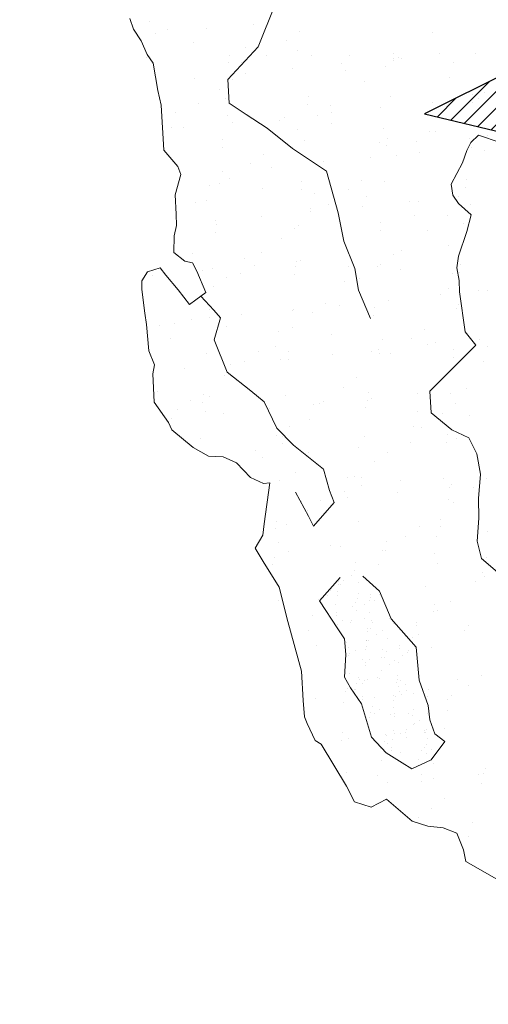
# Model space of a CAD drawing. Units: inches. Extents: x 1986 to 21484, y -1816 to 2016.
# Tile 54 of 85: x 3644.98 to 3651.09, y 1870.8 to 1883.64. Entities that reach past the tile are written whole.
import ezdxf

# ---------------------------------------------------------------- set-up
doc = ezdxf.new("R2010")
doc.units = ezdxf.units.IN
for name, color, linetype, lineweight in [('A-ANNO-DIMS', 2, 'Continuous', 18), ('L-PLNT', 84, 'Continuous', 13), ('vfolhas', 114, 'Continuous', 5)]:
    doc.layers.add(name, color=color, linetype=linetype, lineweight=lineweight)
doc.layers.add('vfolhas2', color=102, linetype='Continuous')
doc.styles.get("Standard").update_dxf_attribs({"font": 'arial.ttf'})
doc.dimstyles.new('ISO-25', dxfattribs={"dimtxt": 8, "dimasz": 2.5, "dimexe": 1.25, "dimexo": 0.625, "dimtad": 1, "dimdec": 1, "dimlunit": 3, "dimtxsty": 'Standard', "dimcen": 2.5, "dimadec": 0, "dimazin": 0, "dimtfac": 1, "dimtdec": 1, "dimtmove": 0, "dimatfit": 3, "dimfxl": 1, "dimarcsym": 0})

# ---------------------------------------------------------------- blocks, each defined once
blk = doc.blocks.new('arbusto_PB_verde_grande')
at = {"layer": 'vfolhas'}
h = blk.add_hatch(dxfattribs=at)
h.set_pattern_fill('ANSI31', color=256, scale=0.05, style=0)
h.set_pattern_definition([(45, (-2446.5133113, 50.986076), (-0.004419417382, 0.004419417382), [])])
h.paths.add_polyline_path([(-0.57219, 0.06233), (-0.7153, 0.10298), (-0.67736, 0.08107), (-0.62769, 0.01536), (-0.56347, -0.04095), (-0.26461, -0.0834), (-0.14874, -0.06595), (-0.10151, -0.05877), (-0.20418, -0.0472), (-0.40279, -0.00339)])
h.paths.add_polyline_path([(-0.56347, -0.04095), (-0.58279, -0.02401), (-0.72992, -0.09726), (-0.4334, -0.1679), (-0.41452, -0.15048), (-0.31518, -0.09101), (-0.26461, -0.0834)])
h.paths.add_polyline_path([(-0.2769, -0.47267), (-0.27429, -0.44776), (-0.16328, -0.25376), (0.02625, -0.03934), (-0.21007, -0.20995), (-0.2672, -0.24466), (-0.36485, -0.35697), (-0.42907, -0.46341), (-0.47586, -0.60425), (-0.37946, -0.57603)])
at = {"layer": 'vfolhas2'}
for p, q in [((-0.58279, -0.02401), (-0.72992, -0.09726)), ((-0.72992, -0.09726), (-0.4334, -0.1679))]:
    blk.add_line(p, q, dxfattribs=at)
blk = doc.blocks.new('PLANT-SHRUB')
for p, q in [((2184.788, 1886.333), (2184.967, 1885.753)), ((2184.967, 1885.753), (2184.886, 1885.62)), ((2184.724, 1885.539), (2184.724, 1885.539)), ((2184.886, 1885.62), (2184.799, 1885.401)), ((2184.551, 1885.444), (2184.551, 1885.444)), ((2184.799, 1885.401), (2184.88, 1885.228)), ((2184.117, 1885.152), (2184.117, 1885.152)), ((2184.88, 1885.228), (2185.013, 1885.078)), ((2183.949, 1885.045), (2183.949, 1885.045)), ((2184.011, 1885.069), (2184.011, 1885.069)), ((2184.062, 1885.039), (2184.062, 1885.039)), ((2185.013, 1885.078), (2185.117, 1884.888)), ((2184.605, 1884.968), (2184.605, 1884.968)), ((2184.813, 1884.94), (2184.813, 1884.94)), ((2185.028, 1884.913), (2185.028, 1884.913)), ((2185.117, 1884.888), (2185.163, 1884.45)), ((2184.526, 1884.674), (2184.526, 1884.674)), ((2184.387, 1884.475), (2184.095, 1884.424)), ((2184.387, 1884.475), (2184.387, 1884.475)), ((2184.654, 1884.389), (2184.387, 1884.475)), ((2184.401, 1884.538), (2184.401, 1884.538)), ((2184.607, 1884.526), (2184.607, 1884.526)), ((2184.68, 1884.594), (2184.68, 1884.594)), ((2184.095, 1884.424), (2184.121, 1884.259)), ((2184.293, 1884.388), (2184.293, 1884.388)), ((2184.377, 1884.377), (2184.377, 1884.377)), ((2184.507, 1884.36), (2184.507, 1884.36)), ((2184.691, 1884.247), (2184.654, 1884.389)), ((2185.163, 1884.45), (2185.382, 1884.392)), ((2185.163, 1884.45), (2185.163, 1884.45)), ((2185.382, 1884.392), (2185.492, 1884.19)), ((2183.986, 1884.299), (2183.986, 1884.299)), ((2184.121, 1884.259), (2184.045, 1884.082)), ((2184.235, 1884.244), (2184.235, 1884.244)), ((2184.302, 1884.287), (2184.302, 1884.287)), ((2184.338, 1884.301), (2184.338, 1884.301)), ((2184.396, 1884.3), (2184.396, 1884.3)), ((2184.755, 1884.006), (2184.691, 1884.247)), ((2185.008, 1884.304), (2185.008, 1884.304)), ((2183.16, 1884.123), (2183.16, 1884.123)), ((2183.368, 1884.095), (2183.368, 1884.095)), ((2183.795, 1884.152), (2183.795, 1884.152)), ((2184.045, 1884.082), (2183.931, 1883.93)), ((2184.17, 1884.146), (2184.17, 1884.146)), ((2184.194, 1884.14), (2184.194, 1884.14)), ((2184.199, 1884.173), (2184.199, 1884.173)), ((2184.209, 1884.162), (2184.209, 1884.162)), ((2184.612, 1884.134), (2184.612, 1884.134)), ((2185.039, 1884.149), (2185.039, 1884.149)), ((2185.492, 1884.19), (2185.428, 1883.971)), ((2183.626, 1884.044), (2183.626, 1884.044)), ((2183.693, 1884.053), (2183.693, 1884.053)), ((2183.977, 1883.99), (2183.977, 1883.99)), ((2184.011, 1884), (2184.011, 1884)), ((2184.146, 1883.993), (2184.146, 1883.993)), ((2184.229, 1883.982), (2184.229, 1883.982)), ((2184.236, 1883.981), (2184.236, 1883.981)), ((2184.359, 1883.965), (2184.359, 1883.965)), ((2184.386, 1883.992), (2184.386, 1883.992)), ((2184.416, 1884.041), (2184.416, 1884.041)), ((2184.444, 1883.954), (2184.444, 1883.954)), ((2184.651, 1884.006), (2184.651, 1884.006)), ((2184.68, 1884.033), (2184.68, 1884.033)), ((2184.755, 1884.006), (2184.755, 1884.006)), ((2184.755, 1883.727), (2184.755, 1884.006)), ((2184.871, 1884.042), (2184.871, 1884.042)), ((2185.428, 1883.971), (2185.296, 1883.345)), ((2183.421, 1883.943), (2183.421, 1883.943)), ((2183.931, 1883.93), (2183.791, 1883.613)), ((2183.861, 1883.843), (2183.861, 1883.843)), ((2184.105, 1883.844), (2184.105, 1883.844)), ((2184.173, 1883.887), (2184.173, 1883.887)), ((2184.183, 1883.832), (2184.183, 1883.832)), ((2184.491, 1883.86), (2184.491, 1883.86)), ((2184.501, 1883.904), (2184.501, 1883.904)), ((2184.576, 1883.936), (2184.576, 1883.936)), ((2184.602, 1883.826), (2184.602, 1883.826)), ((2184.603, 1883.843), (2184.603, 1883.843)), ((2184.659, 1883.926), (2184.659, 1883.926)), ((2184.671, 1883.886), (2184.671, 1883.886)), ((2184.769, 1883.911), (2184.769, 1883.911)), ((2185.312, 1883.84), (2185.312, 1883.84)), ((2183.788, 1883.776), (2183.788, 1883.776)), ((2184.323, 1883.706), (2184.323, 1883.706)), ((2184.352, 1883.733), (2184.352, 1883.733)), ((2184.552, 1883.322), (2184.755, 1883.727)), ((2183.791, 1883.613), (2183.525, 1883.271)), ((2183.967, 1883.682), (2183.967, 1883.682)), ((2183.999, 1883.599), (2183.999, 1883.599)), ((2184.082, 1883.588), (2184.082, 1883.588)), ((2184.212, 1883.571), (2184.212, 1883.571)), ((2184.286, 1883.641), (2184.286, 1883.641)), ((2184.376, 1883.684), (2184.376, 1883.684)), ((2182.834, 1883.54), (2182.834, 1883.54)), ((2182.914, 1883.543), (2182.914, 1883.543)), ((2183.742, 1883.539), (2183.742, 1883.539)), ((2183.96, 1883.529), (2183.96, 1883.529)), ((2183.976, 1883.443), (2183.976, 1883.443)), ((2184.044, 1883.486), (2184.044, 1883.486)), ((2184.079, 1883.537), (2184.079, 1883.537)), ((2184.164, 1883.56), (2184.164, 1883.56)), ((2184.173, 1883.524), (2184.173, 1883.524)), ((2184.429, 1883.542), (2184.429, 1883.542)), ((2184.474, 1883.442), (2184.474, 1883.442)), ((2184.512, 1883.531), (2184.512, 1883.531)), ((2184.542, 1883.485), (2184.542, 1883.485)), ((2184.592, 1883.518), (2184.592, 1883.518)), ((2184.642, 1883.514), (2184.642, 1883.514)), ((2184.983, 1883.534), (2184.983, 1883.534)), ((2185.063, 1883.493), (2185.063, 1883.493)), ((2182.068, 1883.402), (2182.113, 1883.009)), ((2183.39, 1883.411), (2183.39, 1883.411)), ((2183.957, 1883.374), (2183.957, 1883.374)), ((2183.995, 1883.405), (2183.995, 1883.405)), ((2184.025, 1883.432), (2184.025, 1883.432)), ((2184.366, 1883.376), (2184.366, 1883.376)), ((2184.514, 1883.068), (2184.552, 1883.322)), ((2184.989, 1883.425), (2184.989, 1883.425)), ((2185.296, 1883.345), (2185.319, 1883.253)), ((2182.249, 1883.208), (2182.249, 1883.208)), ((2183.525, 1883.271), (2183.512, 1882.777)), ((2183.525, 1883.271), (2183.525, 1883.271)), ((2183.634, 1883.233), (2183.634, 1883.233)), ((2183.659, 1883.241), (2183.659, 1883.241)), ((2183.732, 1883.231), (2183.732, 1883.231)), ((2183.836, 1883.26), (2183.836, 1883.26)), ((2183.851, 1883.204), (2183.851, 1883.204)), ((2183.934, 1883.193), (2183.934, 1883.193)), ((2184.157, 1883.241), (2184.157, 1883.241)), ((2184.163, 1883.216), (2184.163, 1883.216)), ((2184.476, 1883.265), (2184.476, 1883.265)), ((2184.505, 1883.292), (2184.505, 1883.292)), ((2185.319, 1883.253), (2185.244, 1883.022)), ((2182.227, 1883.153), (2182.227, 1883.153)), ((2182.374, 1883.168), (2182.374, 1883.168)), ((2182.792, 1883.137), (2182.792, 1883.137)), ((2183, 1883.109), (2183, 1883.109)), ((2183.042, 1883.093), (2183.042, 1883.093)), ((2183.325, 1883.066), (2183.325, 1883.066)), ((2183.396, 1883.173), (2183.396, 1883.173)), ((2183.472, 1883.151), (2183.472, 1883.151)), ((2183.529, 1883.071), (2183.529, 1883.071)), ((2183.667, 1883.105), (2183.667, 1883.105)), ((2183.697, 1883.132), (2183.697, 1883.132)), ((2183.915, 1883.086), (2183.915, 1883.086)), ((2183.947, 1883.066), (2183.947, 1883.066)), ((2184.064, 1883.176), (2184.064, 1883.176)), ((2184.281, 1883.147), (2184.281, 1883.147)), ((2184.317, 1883.119), (2184.317, 1883.119)), ((2184.356, 1883.068), (2184.356, 1883.068)), ((2184.365, 1883.136), (2184.365, 1883.136)), ((2184.412, 1883.085), (2184.412, 1883.085)), ((2184.476, 1883.134), (2184.476, 1883.134)), ((2184.476, 1882.916), (2184.514, 1883.068)), ((2184.495, 1883.119), (2184.495, 1883.119)), ((2184.514, 1883.068), (2184.514, 1883.068)), ((2184.591, 1883.061), (2184.591, 1883.061)), ((2184.717, 1883.149), (2184.717, 1883.149)), ((2182.113, 1883.009), (2182, 1882.806)), ((2182.059, 1883.046), (2182.059, 1883.046)), ((2182.968, 1883.025), (2182.968, 1883.025)), ((2183.303, 1883.043), (2183.303, 1883.043)), ((2183.847, 1883.043), (2183.847, 1883.043)), ((2183.868, 1882.995), (2183.868, 1882.995)), ((2184.076, 1882.968), (2184.076, 1882.968)), ((2184.148, 1882.965), (2184.148, 1882.965)), ((2184.178, 1882.992), (2184.178, 1882.992)), ((2184.345, 1883.042), (2184.345, 1883.042)), ((2184.548, 1883.041), (2184.548, 1883.041)), ((2185.21, 1882.935), (2185.077, 1882.768)), ((2185.244, 1883.022), (2185.21, 1882.935)), ((2182, 1882.806), (2181.775, 1882.603)), ((2181.81, 1882.811), (2181.81, 1882.811)), ((2182, 1882.806), (2182, 1882.806)), ((2183.53, 1882.841), (2183.53, 1882.841)), ((2183.704, 1882.81), (2183.704, 1882.81)), ((2183.721, 1882.923), (2183.721, 1882.923)), ((2183.787, 1882.799), (2183.787, 1882.799)), ((2183.989, 1882.819), (2183.989, 1882.819)), ((2184.028, 1882.84), (2184.028, 1882.84)), ((2184.153, 1882.908), (2184.153, 1882.908)), ((2184.26, 1882.713), (2184.476, 1882.916)), ((2184.401, 1882.925), (2184.401, 1882.925)), ((2184.944, 1882.853), (2184.944, 1882.853)), ((2182.889, 1882.773), (2182.889, 1882.773)), ((2183.512, 1882.777), (2183.373, 1882.409)), ((2183.512, 1882.777), (2183.512, 1882.777)), ((2183.519, 1882.763), (2183.519, 1882.763)), ((2183.786, 1882.686), (2183.786, 1882.686)), ((2183.85, 1882.692), (2183.85, 1882.692)), ((2183.917, 1882.782), (2183.917, 1882.782)), ((2183.935, 1882.759), (2183.935, 1882.759)), ((2183.937, 1882.758), (2183.937, 1882.758)), ((2184.133, 1882.549), (2184.26, 1882.713)), ((2184.134, 1882.753), (2184.134, 1882.753)), ((2184.17, 1882.674), (2184.17, 1882.674)), ((2184.217, 1882.742), (2184.217, 1882.742)), ((2184.244, 1882.742), (2184.244, 1882.742)), ((2185.077, 1882.768), (2184.829, 1882.474)), ((2181.775, 1882.603), (2181.606, 1882.412)), ((2182.571, 1882.661), (2182.571, 1882.661)), ((2183.711, 1882.615), (2183.711, 1882.615)), ((2183.718, 1882.643), (2183.718, 1882.643)), ((2183.82, 1882.665), (2183.82, 1882.665)), ((2184.108, 1882.397), (2184.133, 1882.549)), ((2184.143, 1882.6), (2184.143, 1882.6)), ((2181.606, 1882.412), (2181.369, 1882.198)), ((2182.511, 1882.539), (2182.511, 1882.539)), ((2183.401, 1882.441), (2183.401, 1882.441)), ((2183.509, 1882.455), (2183.509, 1882.455)), ((2183.556, 1882.415), (2183.556, 1882.415)), ((2183.661, 1882.519), (2183.661, 1882.519)), ((2183.756, 1882.537), (2183.756, 1882.537)), ((2183.899, 1882.44), (2183.899, 1882.44)), ((2183.927, 1882.45), (2183.927, 1882.45)), ((2184.829, 1882.474), (2184.517, 1881.881)), ((2181.348, 1882.292), (2181.348, 1882.292)), ((2182.223, 1882.342), (2182.223, 1882.342)), ((2182.349, 1882.398), (2182.349, 1882.398)), ((2183.371, 1882.403), (2183.371, 1882.403)), ((2183.373, 1882.409), (2183.398, 1882.118)), ((2183.373, 1882.409), (2183.373, 1882.409)), ((2183.493, 1882.364), (2183.493, 1882.364)), ((2183.522, 1882.391), (2183.522, 1882.391)), ((2183.64, 1882.404), (2183.64, 1882.404)), ((2183.656, 1882.285), (2183.656, 1882.285)), ((2183.701, 1882.307), (2183.701, 1882.307)), ((2183.77, 1882.387), (2183.77, 1882.387)), ((2183.772, 1882.31), (2183.772, 1882.31)), ((2183.987, 1882.358), (2183.987, 1882.358)), ((2184.032, 1881.966), (2184.108, 1882.397)), ((2184.07, 1882.347), (2184.07, 1882.347)), ((2184.45, 1882.364), (2184.45, 1882.364)), ((2181.369, 1882.198), (2181.223, 1881.973)), ((2181.556, 1882.265), (2181.556, 1882.265)), ((2181.881, 1882.222), (2181.881, 1882.222)), ((2182.149, 1882.275), (2182.149, 1882.275)), ((2183.589, 1882.242), (2183.589, 1882.242)), ((2183.973, 1882.224), (2183.973, 1882.224)), ((2184.003, 1882.251), (2184.003, 1882.251)), ((2181.736, 1882.045), (2181.736, 1882.045)), ((2181.784, 1882.041), (2181.784, 1882.041)), ((2181.904, 1882.152), (2181.904, 1882.152)), ((2182.423, 1882.15), (2182.423, 1882.15)), ((2182.631, 1882.123), (2182.631, 1882.123)), ((2182.956, 1882.08), (2182.956, 1882.08)), ((2182.981, 1882.043), (2182.981, 1882.043)), ((2183.149, 1882.15), (2183.149, 1882.15)), ((2183.398, 1882.118), (2183.398, 1882.118)), ((2183.498, 1882.147), (2183.498, 1882.147)), ((2183.77, 1882.04), (2183.77, 1882.04)), ((2183.814, 1882.078), (2183.814, 1882.078)), ((2183.917, 1882.142), (2183.917, 1882.142)), ((2184.225, 1882.04), (2184.225, 1882.04)), ((2184.394, 1882.148), (2184.394, 1882.148)), ((2181.223, 1881.973), (2181.155, 1881.748)), ((2181.751, 1881.91), (2181.751, 1881.91)), ((2182.864, 1882.002), (2182.864, 1882.002)), ((2183.351, 1881.924), (2183.351, 1881.924)), ((2183.424, 1881.991), (2183.424, 1881.991)), ((2183.499, 1882.009), (2183.499, 1882.009)), ((2183.622, 1881.992), (2183.622, 1881.992)), ((2183.626, 1881.928), (2184.032, 1881.966)), ((2183.675, 1881.951), (2183.675, 1881.951)), ((2183.691, 1881.999), (2183.691, 1881.999)), ((2183.707, 1881.981), (2183.707, 1881.981)), ((2183.839, 1881.964), (2183.839, 1881.964)), ((2183.91, 1881.989), (2183.91, 1881.989)), ((2184.032, 1881.938), (2184.032, 1881.938)), ((2184.517, 1881.881), (2184.292, 1881.477)), ((2181.155, 1881.748), (2181.245, 1881.523)), ((2181.277, 1881.641), (2181.277, 1881.641)), ((2180.944, 1881.54), (2180.944, 1881.54)), ((2181.245, 1881.523), (2181.29, 1881.174)), ((2181.33, 1881.524), (2181.33, 1881.524)), ((2181.404, 1881.591), (2181.404, 1881.591)), ((2182.188, 1881.538), (2182.188, 1881.538)), ((2182.323, 1881.628), (2182.323, 1881.628)), ((2182.953, 1881.559), (2182.953, 1881.559)), ((2183.346, 1881.633), (2183.346, 1881.633)), ((2183.433, 1881.536), (2183.433, 1881.536)), ((2184.425, 1881.594), (2184.425, 1881.594)), ((2184.292, 1881.477), (2184.216, 1881.087)), ((2180.737, 1881.266), (2180.737, 1881.266)), ((2180.979, 1881.306), (2180.979, 1881.306)), ((2181.187, 1881.278), (2181.187, 1881.278)), ((2181.759, 1881.271), (2181.759, 1881.271)), ((2180.337, 1881.154), (2180.337, 1881.154)), ((2180.932, 1881.159), (2180.932, 1881.159)), ((2181.29, 1881.174), (2181.11, 1880.96)), ((2181.512, 1881.235), (2181.512, 1881.235)), ((2181.582, 1881.151), (2181.582, 1881.151)), ((2182.055, 1881.164), (2182.055, 1881.164)), ((2182.263, 1881.137), (2182.263, 1881.137)), ((2182.532, 1881.173), (2182.532, 1881.173)), ((2182.605, 1881.241), (2182.605, 1881.241)), ((2182.826, 1881.149), (2182.826, 1881.149)), ((2182.839, 1881.232), (2182.839, 1881.232)), ((2182.952, 1881.008), (2183.014, 1881.159)), ((2183.014, 1881.159), (2183.422, 1881.204)), ((2183.014, 1881.159), (2183.014, 1881.159)), ((2183.422, 1881.204), (2183.378, 1881.062)), ((2183.885, 1881.219), (2183.885, 1881.219)), ((2184.071, 1881.147), (2184.071, 1881.147)), ((2184.154, 1881.208), (2184.154, 1881.208)), ((2180.169, 1881.046), (2180.169, 1881.046)), ((2181.413, 1881.044), (2181.413, 1881.044)), ((2182.588, 1881.094), (2182.588, 1881.094)), ((2182.658, 1881.042), (2182.658, 1881.042)), ((2182.819, 1880.751), (2182.952, 1881.008)), ((2183.131, 1881.022), (2183.131, 1881.022)), ((2183.378, 1881.062), (2183.289, 1880.716)), ((2183.902, 1881.04), (2183.902, 1881.04)), ((2184.216, 1881.087), (2184.176, 1880.891)), ((2180.173, 1880.91), (2180.173, 1880.91)), ((2180.262, 1880.928), (2180.242, 1880.708)), ((2181.11, 1880.96), (2180.262, 1880.928)), ((2181.11, 1880.96), (2181.11, 1880.96)), ((2181.252, 1880.871), (2181.252, 1880.871)), ((2183.339, 1880.995), (2183.339, 1880.995)), ((2183.664, 1880.952), (2183.664, 1880.952)), ((2183.807, 1880.89), (2183.807, 1880.89)), ((2184.176, 1880.891), (2183.986, 1880.834)), ((2180.511, 1880.773), (2180.511, 1880.773)), ((2180.585, 1880.841), (2180.585, 1880.841)), ((2182.134, 1880.809), (2182.134, 1880.809)), ((2182.298, 1880.858), (2182.298, 1880.858)), ((2182.889, 1880.253), (2182.819, 1880.751)), ((2183.321, 1880.863), (2183.321, 1880.863)), ((2183.733, 1880.822), (2183.733, 1880.822)), ((2183.986, 1880.834), (2183.87, 1880.741)), ((2180.242, 1880.708), (2179.942, 1880.278)), ((2183.87, 1880.741), (2183.449, 1880.401)), ((2179.665, 1880.51), (2179.665, 1880.51)), ((2180.621, 1880.539), (2180.621, 1880.539)), ((2180.712, 1880.496), (2180.712, 1880.496)), ((2181.734, 1880.501), (2181.734, 1880.501)), ((2181.786, 1880.49), (2181.786, 1880.49)), ((2181.866, 1880.537), (2181.866, 1880.537)), ((2183.11, 1880.535), (2183.11, 1880.535)), ((2179.743, 1880.434), (2179.743, 1880.434)), ((2180.068, 1880.391), (2180.068, 1880.391)), ((2180.113, 1880.409), (2180.113, 1880.409)), ((2181.712, 1880.422), (2181.712, 1880.422)), ((2182.813, 1880.462), (2182.813, 1880.462)), ((2183.335, 1880.458), (2183.335, 1880.458)), ((2183.449, 1880.401), (2183.518, 1880.349)), ((2179.942, 1880.278), (2179.842, 1880.168)), ((2180.611, 1880.319), (2180.611, 1880.319)), ((2180.819, 1880.292), (2180.819, 1880.292)), ((2181.144, 1880.249), (2181.144, 1880.249)), ((2182.898, 1879.943), (2182.889, 1880.253)), ((2183.518, 1880.349), (2183.588, 1880.176)), ((2179.842, 1880.168), (2179.752, 1880.028)), ((2180.014, 1880.153), (2180.014, 1880.153)), ((2180.147, 1880.14), (2180.147, 1880.14)), ((2181.227, 1880.101), (2181.227, 1880.101)), ((2181.259, 1880.151), (2181.259, 1880.151)), ((2181.686, 1880.178), (2181.686, 1880.178)), ((2181.895, 1880.15), (2181.895, 1880.15)), ((2182.219, 1880.108), (2182.219, 1880.108)), ((2182.504, 1880.148), (2182.504, 1880.148)), ((2182.987, 1880.139), (2182.987, 1880.139)), ((2183.588, 1880.176), (2183.588, 1879.911)), ((2179.752, 1880.028), (2179.632, 1879.928)), ((2179.692, 1880.023), (2179.692, 1880.023)), ((2179.765, 1880.09), (2179.765, 1880.09)), ((2179.846, 1880.046), (2179.846, 1880.046)), ((2181.09, 1880.043), (2181.09, 1880.043)), ((2181.315, 1880.058), (2181.315, 1880.058)), ((2182.273, 1880.088), (2182.273, 1880.088)), ((2182.335, 1880.041), (2182.335, 1880.041)), ((2182.762, 1880.036), (2182.762, 1880.036)), ((2182.914, 1880.072), (2182.914, 1880.072)), ((2182.97, 1880.009), (2182.97, 1880.009)), ((2183.295, 1880.092), (2183.295, 1880.092)), ((2183.58, 1880.039), (2183.58, 1880.039)), ((2179.632, 1879.928), (2179.331, 1879.768)), ((2179.632, 1879.928), (2179.632, 1879.928)), ((2182.782, 1879.579), (2182.898, 1879.943)), ((2183.295, 1879.966), (2183.295, 1879.966)), ((2183.588, 1879.911), (2183.663, 1879.738)), ((2179.331, 1879.768), (2179.141, 1879.648)), ((2179.64, 1879.739), (2179.64, 1879.739)), ((2180.686, 1879.726), (2180.686, 1879.726)), ((2181.028, 1879.737), (2180.888, 1879.358)), ((2180.967, 1879.739), (2180.967, 1879.739)), ((2181.709, 1879.731), (2181.709, 1879.731)), ((2183.663, 1879.738), (2183.795, 1879.6)), ((2179.141, 1879.648), (2179.161, 1879.428)), ((2179.294, 1879.658), (2179.294, 1879.658)), ((2180.893, 1879.672), (2180.893, 1879.672)), ((2182.516, 1879.707), (2182.516, 1879.707)), ((2182.788, 1879.692), (2182.788, 1879.692)), ((2183.795, 1879.6), (2183.865, 1879.381)), ((2179.054, 1879.541), (2179.054, 1879.541)), ((2179.166, 1879.475), (2179.166, 1879.475)), ((2180.298, 1879.539), (2180.298, 1879.539)), ((2181.543, 1879.536), (2181.543, 1879.536)), ((2182.809, 1879.357), (2182.782, 1879.579)), ((2182.787, 1879.534), (2182.787, 1879.534)), ((2178.946, 1879.34), (2178.946, 1879.34)), ((2179.1, 1879.365), (2179.1, 1879.365)), ((2179.161, 1879.428), (2179.141, 1879.298)), ((2179.374, 1879.447), (2179.374, 1879.447)), ((2179.699, 1879.404), (2179.699, 1879.404)), ((2180.122, 1879.37), (2180.122, 1879.37)), ((2180.242, 1879.333), (2180.242, 1879.333)), ((2180.888, 1879.358), (2180.729, 1879.119)), ((2181.202, 1879.331), (2181.202, 1879.331)), ((2182.168, 1879.389), (2182.168, 1879.389)), ((2182.871, 1878.967), (2182.809, 1879.357)), ((2183.717, 1879.356), (2183.717, 1879.356)), ((2183.865, 1879.381), (2183.909, 1879.023)), ((2178.361, 1878.959), (2178.221, 1879.219)), ((2178.873, 1879.272), (2178.873, 1879.272)), ((2179.141, 1879.298), (2179.061, 1879.179)), ((2180.45, 1879.306), (2180.45, 1879.306)), ((2180.495, 1879.307), (2180.495, 1879.307)), ((2180.775, 1879.263), (2180.775, 1879.263)), ((2182.095, 1879.321), (2182.095, 1879.321)), ((2182.248, 1879.317), (2182.248, 1879.317)), ((2183.27, 1879.322), (2183.27, 1879.322)), ((2178.447, 1879.154), (2178.447, 1879.154)), ((2178.761, 1879.079), (2178.611, 1878.999)), ((2179.061, 1879.179), (2178.761, 1879.079)), ((2179.691, 1879.152), (2179.691, 1879.152)), ((2180.729, 1879.119), (2180.589, 1878.76)), ((2180.936, 1879.15), (2180.936, 1879.15)), ((2181.318, 1879.191), (2181.318, 1879.191)), ((2181.526, 1879.164), (2181.526, 1879.164)), ((2181.851, 1879.121), (2181.851, 1879.121)), ((2182.181, 1879.148), (2182.181, 1879.148)), ((2183.425, 1879.145), (2183.425, 1879.145)), ((2178.278, 1879.047), (2178.278, 1879.047)), ((2178.501, 1878.959), (2178.361, 1878.959)), ((2178.611, 1878.999), (2178.501, 1878.959)), ((2178.536, 1879.008), (2178.536, 1879.008)), ((2179.523, 1879.045), (2179.523, 1879.045)), ((2179.615, 1878.969), (2179.615, 1878.969)), ((2180.148, 1878.989), (2180.148, 1878.989)), ((2180.661, 1878.956), (2180.661, 1878.956)), ((2180.768, 1879.042), (2180.768, 1879.042)), ((2181.684, 1878.961), (2181.684, 1878.961)), ((2181.697, 1878.957), (2181.697, 1878.957)), ((2182.012, 1879.04), (2182.012, 1879.04)), ((2182.394, 1879.05), (2182.394, 1879.05)), ((2182.602, 1879.022), (2182.602, 1879.022)), ((2182.702, 1878.542), (2182.871, 1878.967)), ((2182.927, 1878.98), (2182.927, 1878.98)), ((2183.257, 1879.038), (2183.257, 1879.038)), ((2183.296, 1878.97), (2183.296, 1878.97)), ((2183.37, 1879.038), (2183.37, 1879.038)), ((2183.909, 1879.023), (2183.877, 1878.92)), ((2178.475, 1878.907), (2178.475, 1878.907)), ((2180.074, 1878.921), (2180.074, 1878.921)), ((2182.763, 1878.922), (2182.763, 1878.922)), ((2183.47, 1878.908), (2183.47, 1878.908)), ((2183.678, 1878.881), (2183.678, 1878.881)), ((2183.809, 1878.909), (2183.809, 1878.909)), ((2183.877, 1878.92), (2183.831, 1878.602)), ((2180.589, 1878.76), (2180.389, 1878.441)), ((2177.93, 1878.603), (2177.93, 1878.603)), ((2178.028, 1878.608), (2178.028, 1878.608)), ((2178.127, 1878.589), (2178.127, 1878.589)), ((2178.255, 1878.56), (2178.255, 1878.56)), ((2179.075, 1878.595), (2179.075, 1878.595)), ((2180.097, 1878.6), (2180.097, 1878.6)), ((2181.176, 1878.561), (2181.176, 1878.561)), ((2181.275, 1878.57), (2181.275, 1878.57)), ((2181.349, 1878.638), (2181.349, 1878.638)), ((2182.898, 1878.606), (2182.898, 1878.606)), ((2183.831, 1878.602), (2183.591, 1878.317)), ((2178.053, 1878.521), (2178.053, 1878.521)), ((2178.731, 1878.54), (2178.731, 1878.54)), ((2178.798, 1878.488), (2178.798, 1878.488)), ((2179.006, 1878.461), (2179.006, 1878.461)), ((2179.676, 1878.557), (2179.676, 1878.557)), ((2179.975, 1878.538), (2179.975, 1878.538)), ((2180.389, 1878.441), (2180.13, 1877.943)), ((2180.389, 1878.441), (2180.389, 1878.441)), ((2181.22, 1878.536), (2181.22, 1878.536)), ((2182.223, 1878.547), (2182.223, 1878.547)), ((2182.445, 1878.391), (2182.702, 1878.542)), ((2182.465, 1878.533), (2182.465, 1878.533)), ((2183.245, 1878.552), (2183.245, 1878.552)), ((2183.709, 1878.531), (2183.709, 1878.531)), ((2179.331, 1878.418), (2179.331, 1878.418)), ((2179.874, 1878.347), (2179.874, 1878.347)), ((2180.082, 1878.319), (2180.082, 1878.319)), ((2182.44, 1878.258), (2182.445, 1878.391)), ((2183.591, 1878.317), (2183.494, 1878.246)), ((2178.51, 1878.238), (2178.51, 1878.238)), ((2179.328, 1878.238), (2179.328, 1878.238)), ((2179.59, 1878.199), (2179.59, 1878.199)), ((2180.407, 1878.277), (2180.407, 1878.277)), ((2180.636, 1878.186), (2180.636, 1878.186)), ((2180.878, 1878.206), (2180.878, 1878.206)), ((2180.949, 1878.205), (2180.949, 1878.205)), ((2181.158, 1878.178), (2181.158, 1878.178)), ((2181.658, 1878.191), (2181.658, 1878.191)), ((2182.44, 1878.008), (2182.44, 1878.258)), ((2182.477, 1878.22), (2182.477, 1878.22)), ((2182.551, 1878.287), (2182.551, 1878.287)), ((2183.494, 1878.246), (2183.423, 1878.064)), ((2177.656, 1878.157), (2177.656, 1878.157)), ((2177.956, 1878.046), (2177.956, 1878.046)), ((2178.124, 1878.154), (2178.124, 1878.154)), ((2179.255, 1878.171), (2179.255, 1878.171)), ((2179.369, 1878.151), (2179.369, 1878.151)), ((2180.613, 1878.149), (2180.613, 1878.149)), ((2181.482, 1878.135), (2181.482, 1878.135)), ((2181.858, 1878.147), (2181.858, 1878.147)), ((2182.025, 1878.063), (2182.025, 1878.063)), ((2182.738, 1878.152), (2182.738, 1878.152)), ((2183.103, 1878.144), (2183.103, 1878.144)), ((2183.423, 1878.064), (2183.209, 1877.792)), ((2179.2, 1878.044), (2179.2, 1878.044)), ((2180.13, 1877.943), (2180.25, 1877.424)), ((2180.445, 1878.042), (2180.445, 1878.042)), ((2181.689, 1878.039), (2181.689, 1878.039)), ((2182.233, 1878.036), (2182.233, 1878.036)), ((2182.359, 1878.019), (2182.255, 1877.734)), ((2182.359, 1878.019), (2182.359, 1878.019)), ((2182.521, 1877.998), (2182.359, 1878.019)), ((2182.625, 1877.986), (2182.521, 1877.998)), ((2182.558, 1877.993), (2182.558, 1877.993)), ((2182.599, 1877.747), (2182.625, 1877.986)), ((2182.934, 1878.037), (2182.934, 1878.037)), ((2183.101, 1877.922), (2183.101, 1877.922)), ((2178.003, 1877.838), (2178.003, 1877.838)), ((2178.857, 1877.806), (2178.857, 1877.806)), ((2179.049, 1877.825), (2179.049, 1877.825)), ((2180.072, 1877.829), (2180.072, 1877.829)), ((2180.456, 1877.82), (2180.456, 1877.82)), ((2180.53, 1877.887), (2180.53, 1877.887)), ((2181.151, 1877.791), (2181.151, 1877.791)), ((2182.079, 1877.855), (2182.079, 1877.855)), ((2183.209, 1877.792), (2183.124, 1877.669)), ((2182.197, 1877.777), (2182.197, 1877.777)), ((2182.255, 1877.734), (2182.223, 1877.617)), ((2182.586, 1877.494), (2182.599, 1877.747)), ((2182.599, 1877.747), (2182.599, 1877.747)), ((2183.124, 1877.669), (2182.943, 1877.416)), ((2177.886, 1877.574), (2177.886, 1877.574)), ((2178.408, 1877.539), (2178.408, 1877.539)), ((2179.653, 1877.537), (2179.653, 1877.537)), ((2180.897, 1877.535), (2180.897, 1877.535)), ((2181.731, 1877.537), (2181.731, 1877.537)), ((2182.142, 1877.532), (2182.142, 1877.532)), ((2182.223, 1877.617), (2182.281, 1877.533)), ((2182.281, 1877.533), (2182.307, 1877.351)), ((2178.429, 1877.502), (2178.429, 1877.502)), ((2178.436, 1877.42), (2178.436, 1877.42)), ((2178.485, 1877.468), (2178.485, 1877.468)), ((2178.509, 1877.487), (2178.509, 1877.487)), ((2178.637, 1877.475), (2178.637, 1877.475)), ((2178.962, 1877.432), (2178.962, 1877.432)), ((2179.565, 1877.429), (2179.565, 1877.429)), ((2180.058, 1877.455), (2180.058, 1877.455)), ((2180.25, 1877.424), (2180.31, 1877.006)), ((2180.611, 1877.416), (2180.611, 1877.416)), ((2181.633, 1877.421), (2181.633, 1877.421)), ((2181.658, 1877.469), (2181.658, 1877.469)), ((2182.573, 1877.377), (2182.586, 1877.494)), ((2182.586, 1877.494), (2182.586, 1877.494)), ((2182.943, 1877.416), (2182.865, 1877.338)), ((2179.505, 1877.36), (2179.505, 1877.36)), ((2179.713, 1877.333), (2179.713, 1877.333)), ((2180.038, 1877.29), (2180.038, 1877.29)), ((2182.307, 1877.351), (2182.158, 1877.196)), ((2182.573, 1877.377), (2182.573, 1877.377)), ((2182.729, 1877.3), (2182.573, 1877.377)), ((2182.713, 1877.382), (2182.713, 1877.382)), ((2182.865, 1877.338), (2182.729, 1877.3)), ((2179.046, 1877.15), (2179.046, 1877.15)), ((2180.291, 1877.148), (2180.291, 1877.148)), ((2180.581, 1877.219), (2180.581, 1877.219)), ((2180.789, 1877.191), (2180.789, 1877.191)), ((2181.114, 1877.149), (2181.114, 1877.149)), ((2181.535, 1877.146), (2181.535, 1877.146)), ((2182.158, 1877.196), (2182.04, 1877.12)), ((2182.158, 1877.196), (2182.158, 1877.196)), ((2178.877, 1877.043), (2178.877, 1877.043)), ((2179.024, 1877.054), (2179.024, 1877.054)), ((2179.637, 1877.069), (2179.637, 1877.069)), ((2179.711, 1877.137), (2179.711, 1877.137)), ((2180.047, 1877.059), (2180.047, 1877.059)), ((2180.122, 1877.041), (2180.122, 1877.041)), ((2181.126, 1877.02), (2181.126, 1877.02)), ((2181.26, 1877.105), (2181.26, 1877.105)), ((2181.367, 1877.039), (2181.367, 1877.039)), ((2181.657, 1877.077), (2181.657, 1877.077)), ((2182.04, 1877.12), (2181.942, 1877.01)), ((2180.31, 1877.006), (2180.389, 1876.687)), ((2181.942, 1877.01), (2181.78, 1876.816)), ((2180.912, 1876.786), (2180.912, 1876.786)), ((2181.78, 1876.816), (2181.547, 1876.673)), ((2179.239, 1876.705), (2179.239, 1876.705)), ((2179.54, 1876.659), (2179.54, 1876.659)), ((2180.389, 1876.687), (2180.449, 1876.428)), ((2180.586, 1876.646), (2180.586, 1876.646)), ((2180.839, 1876.718), (2180.839, 1876.718)), ((2181.547, 1876.673), (2181.501, 1876.57)), ((2179.33, 1876.536), (2179.33, 1876.536)), ((2180.574, 1876.534), (2180.574, 1876.534)), ((2181.501, 1876.57), (2181.488, 1876.291)), ((2180.449, 1876.428), (2180.25, 1876.189)), ((2180.449, 1876.428), (2180.449, 1876.428)), ((2179.137, 1876.374), (2179.137, 1876.374)), ((2179.345, 1876.347), (2179.345, 1876.347)), ((2179.67, 1876.304), (2179.67, 1876.304)), ((2180.021, 1876.289), (2180.021, 1876.289)), ((2180.441, 1876.354), (2180.441, 1876.354)), ((2181.101, 1876.25), (2181.101, 1876.25)), ((2181.488, 1876.291), (2181.112, 1875.837)), ((2179.671, 1876.149), (2179.129, 1875.898)), ((2180.25, 1876.189), (2179.671, 1876.149)), ((2179.671, 1876.149), (2179.671, 1876.149)), ((2179.968, 1876.147), (2179.968, 1876.147)), ((2180.212, 1876.233), (2180.212, 1876.233)), ((2180.25, 1876.189), (2180.25, 1876.189)), ((2180.421, 1876.205), (2180.421, 1876.205)), ((2180.745, 1876.162), (2180.745, 1876.162)), ((2181.212, 1876.145), (2181.212, 1876.145)), ((2179.799, 1876.04), (2179.799, 1876.04)), ((2180.093, 1876.035), (2180.093, 1876.035)), ((2181.044, 1876.038), (2181.044, 1876.038)), ((2179.514, 1875.889), (2179.514, 1875.889)), ((2180.019, 1875.968), (2180.019, 1875.968)), ((2180.561, 1875.876), (2180.561, 1875.876)), ((2181.112, 1875.837), (2181.015, 1875.669)), ((2181.112, 1875.837), (2181.112, 1875.837)), ((2181.015, 1875.669), (2180.813, 1875.367)), ((2179.996, 1875.519), (2179.996, 1875.519)), ((2180.252, 1875.533), (2180.252, 1875.533)), ((2180.813, 1875.367), (2180.794, 1875.231)), ((2180.794, 1875.231), (2180.729, 1875.049)), ((2180.823, 1875.252), (2180.823, 1875.252)), ((2180.377, 1875.176), (2180.377, 1875.176)), ((2180.535, 1875.106), (2180.535, 1875.106)), ((2180.729, 1875.049), (2180.697, 1874.868)), ((2180.721, 1875.037), (2180.721, 1875.037)), ((2180.475, 1874.934), (2180.475, 1874.934)), ((2180.697, 1874.868), (2180.638, 1874.732))]:
    blk.add_line(p, q)
blk = doc.blocks.new('*D96')
at = {"layer": 'A-ANNO-DIMS', "color": 0, "lineweight": -2, "transparency": 16777216}
for p, q in [((3539.82, 1864.464), (3539.82, 1858.215)), ((3577.115, 1864.464), (3577.115, 1858.215)), ((3542.32, 1859.465), (3574.615, 1859.465)), ((3577.115, 1859.465), (3648.265, 1859.465))]:
    blk.add_line(p, q, dxfattribs=at)
at = {"layer": 'A-ANNO-DIMS', "color": 0, "transparency": 16777216}
for points in [[(3542.32, 1859.882), (3542.32, 1859.048), (3539.82, 1859.465)], [(3574.615, 1859.882), (3574.615, 1859.048), (3577.115, 1859.465)]]:
    blk.add_solid(points, dxfattribs=at)
at = {"layer": 'Defpoints', "color": 0, "transparency": 16777216}
for p in [(3539.82, 1865.089), (3577.115, 1865.089), (3577.115, 1859.465)]:
    blk.add_point(p, dxfattribs=at)
at = {"layer": 'A-ANNO-DIMS', "color": 0, "transparency": 16777216, "insert": (3613.94, 1864.229), "char_height": 8, "attachment_point": 5}
blk.add_mtext('3\'-1 1/2" TYP.', dxfattribs=at)

msp = doc.modelspace()

# ---------------------------------------------------------------- block references
at = {"layer": 'L-PLNT', "rotation": 223.1883365522388}
msp.add_blockref('PLANT-SHRUB', (3953.27, 4742.965), dxfattribs=at)
at = {"layer": 'L-PLNT', "xscale": 24.60366729364114, "yscale": 24.60366729364114, "zscale": 24.60366729364114}
msp.add_blockref('arbusto_PB_verde_grande', (3668.218, 1884.805), dxfattribs=at)

# ---------------------------------------------------------------- dimensions: what is measured, and where the dimension line sits
at = {"layer": 'A-ANNO-DIMS'}
dim = msp.add_linear_dim(base=(3577.115, 1859.465), p1=(3539.82, 1865.089), p2=(3577.115, 1865.089), text='<> TYP.', dimstyle='ISO-25', override={"dimdec": 1, "dimrnd": 0, "dimzin": 1, "dimlunit": 4, "dimfrac": 2}, dxfattribs=at)
dim.commit()
dim.dimension.update_dxf_attribs({"geometry": '*D96', "text_midpoint": (3613.94, 1864.229)})

doc.saveas('drawing.dxf')
